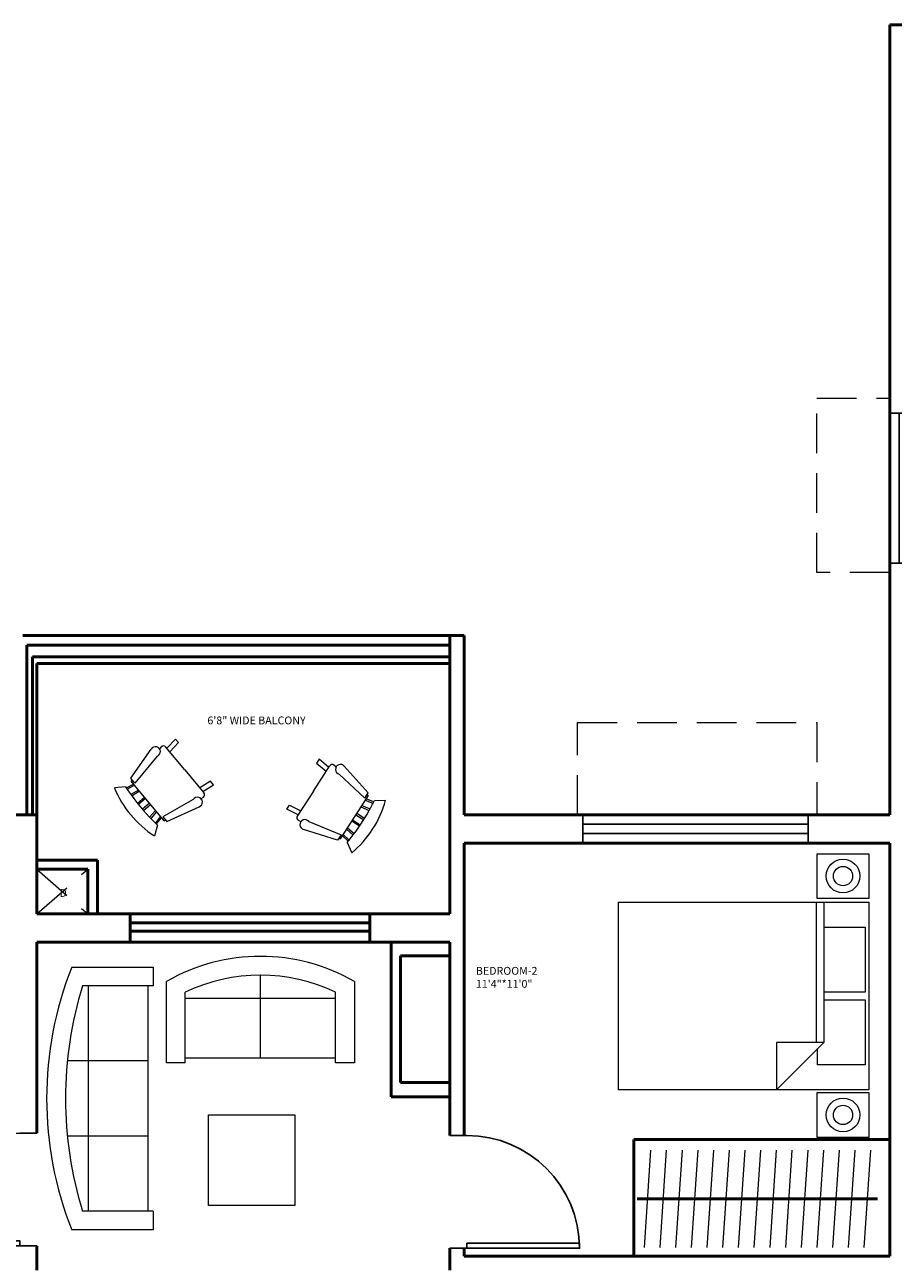
# Model space of a CAD drawing. Units: inches. Extents: x 291 to 2631, y 456 to 2623.
# Tile 16 of 22: x 1696 to 1974, y 2022 to 2418. Entities that reach past the tile are written whole.
import ezdxf

# ---------------------------------------------------------------- set-up
doc = ezdxf.new("R2010")
doc.units = ezdxf.units.IN
doc.linetypes.add('DASHED', pattern=[19.05, 12.7, -6.35])
for name, color, linetype, lineweight in [('A-ANNO-TEXT', 3, 'Continuous', 25), ('A-AREA-IDEN', 7, 'Continuous', 25), ('A-DOOR', 3, 'Continuous', 25), ('A-FLOR-OVHD', 1, 'DASHED', 18), ('A-FURN', 8, 'Continuous', 18), ('A-GLAZ', 4, 'Continuous', 25), ('A-WALL', 7, 'Continuous', 50)]:
    doc.layers.add(name, color=color, linetype=linetype, lineweight=lineweight)
doc.styles.get("Standard").update_dxf_attribs({"font": 'arial.ttf'})

# ---------------------------------------------------------------- blocks, each defined once
blk = doc.blocks.new('*U2')
for p, q in [((0, 0), (0, -6)), ((40, 0), (40, -6))]:
    blk.add_line(p, q)
blk.add_lwpolyline([(0, 0), (0, 40), (1.75, 40), (1.75, 0)], close=True)
blk.add_arc((0, 0), 40, 0, 90)
blk = doc.blocks.new('Bed - Queen')
for p, q in [((0, -80.00003), (0, 0)), ((0, 0), (59.99999, 0)), ((59.99999, 0), (59.99999, -80.00003)), ((7.99999, -1.2), (28.79998, -1.2)), ((7.99999, -14.4), (7.99999, -1.2)), ((28.79998, -1.2), (28.79998, -14.4)), ((31.19999, -1.2), (51.99999, -1.2)), ((31.19999, -14.4), (31.19999, -1.2)), ((51.99999, -1.2), (51.99999, -16.4)), ((0, -14.4), (44.8, -14.4)), ((59.99999, -29.6), (44.8, -14.4)), ((44.8, -14.4), (44.8, -29.6)), ((44.8, -16.8), (0, -16.8)), ((51.99999, -16.4), (46.79936, -16.4)), ((44.8, -29.6), (59.99999, -29.6)), ((59.99999, -80.00003), (0, -80.00003))]:
    blk.add_line(p, q)
blk = doc.blocks.new('Chair - Rocking')
for p, q in [((-8, -4.5), (-10, -1.5)), ((8, -4.5), (10, -1.5)), ((-9, -7.5), (-12, -18.49999)), ((-7, -7.5), (-9, -7.5)), ((-9, -18.49999), (-7, -7.5)), ((-8.23428, -6.99939), (-8.3093, -7.47958)), ((-8.23041, -7), (8.23915, -7)), ((-7.5, -4.5), (-7, -7)), ((-6.5, -7), (-7.02225, -4.43)), ((-4.5, -7), (-4.96674, -4.19951)), ((-4, -7), (-4.40532, -4.16272)), ((-1.5, -4.05012), (-1.5, -7)), ((-1, -7), (-1, -4.05012)), ((1, -7), (1, -4.04655)), ((1.5, -4.05012), (1.5, -7)), ((4, -7), (4.40187, -4.18694)), ((4.5, -7), (4.96761, -4.19437)), ((6.5, -7), (7, -4.4057)), ((7.5, -4.5), (7, -7)), ((7, -7.5), (9, -7.5)), ((9, -18.49999), (7, -7.5)), ((8.31071, -7.48854), (8.23449, -7.00073)), ((9, -7.5), (12, -18.49999)), ((-10.36644, -20.64523), (-10.5, -21.49999)), ((-9, -22.49999), (-9.5, -26.49999)), ((0, -22.49999), (-9.5, -22.49999)), ((-8, -26.49999), (-7.5, -22.49999)), ((0, -22.49999), (9.5, -22.49999)), ((8, -26.49999), (7.5, -22.49999)), ((9, -22.49999), (9.5, -26.49999)), ((10.5, -21.49999), (10.3575, -20.58798)), ((-9.5, -26.49999), (-8, -26.49999)), ((9.5, -26.49999), (8, -26.49999))]:
    blk.add_line(p, q)
for centre, radius, start, end in [((0, -34.08333), 34.08333, 72.93847, 107.0615), ((0, -68.25004), 64.25, 93.92211, 97.15267), ((0, -68.25004), 64.25, 82.84733, 93.92211), ((-10.5, -18.99999), 1.58114, 161.5651, 18.43495), ((10.5, -18.99999), 1.58114, 161.5651, 18.43495), ((-9.5, -21.49999), 1, 180, 270), ((9.5, -21.49999), 1, 270, 0)]:
    blk.add_arc(centre, radius, start, end)
blk = doc.blocks.new('Sofa - Roundback 7 ft.')
for p, q in [((-12.00002, -32.4421), (-12.00003, -6.5971)), ((11.99997, -32.4421), (11.99998, -6.5971)), ((-36.000027, -34), (-36.000027, -11.4696)), ((35.99998, -34), (35.99998, -11.4696)), ((-35.999844, -13.3819), (35.9998, -13.3819)), ((-36.000027, -32.4421), (35.99998, -32.4421))]:
    blk.add_line(p, q)
for points in [[(-36.000027, -34), (-42.000027, -34), (-42.000027, -8)], [(41.99998, -8), (41.99998, -34), (35.99998, -34)]]:
    blk.add_lwpolyline(points)
for centre, radius, start, end in [((0, -114.25), 114.25, 68.43141, 111.5686), ((-0.00001, -127.1968), 121.1968, 72.72033, 107.2797)]:
    blk.add_arc(centre, radius, start, end)
blk = doc.blocks.new('Sofa - Roundback Loveseat 5 ft.')
for p, q in [((0, -32.44198), (0, -5.99998)), ((-24, -33.99998), (-24, -11.46958)), ((24.00004, -33.99998), (24.00004, -11.46958)), ((-23.9998, -13.38178), (23.99986, -13.38178)), ((-24, -32.44198), (24.00004, -32.44198))]:
    blk.add_line(p, q)
for points in [[(-24, -33.99998), (-30, -33.99998), (-30, -7.99998)], [(30.00004, -7.99998), (30.00004, -33.99998), (24.00004, -33.99998)]]:
    blk.add_lwpolyline(points)
for centre, radius, start, end in [((0, -60.24998), 60.24998, 60.13715, 119.8628), ((0, -61.38438), 55.38444, 64.32083, 115.6792)]:
    blk.add_arc(centre, radius, start, end)
blk = doc.blocks.new('WIN-1800')
for p, q in [((0, 9), (72, 9)), ((0, 0), (0, 9)), ((72, 9), (72, 0)), ((0, 6), (72, 6)), ((72, 3), (0, 3)), ((72, 0), (0, 0))]:
    blk.add_line(p, q)
blk = doc.blocks.new('WIN-1200')
for p, q in [((0, 0), (0, 48)), ((0, 48), (9, 48)), ((3, 0), (3, 48)), ((6, 48), (6, 0)), ((9, 48), (9, 0)), ((9, 0), (0, 0))]:
    blk.add_line(p, q)

msp = doc.modelspace()

# ---------------------------------------------------------------- linework, layer by layer
at = {"layer": 'A-FLOR-OVHD'}
for p, q in [((1949.18, 2242.68), (1949.18, 2298.43)), ((1949.18, 2298.43), (1972.49, 2298.43)), ((1972.49, 2242.68), (1949.18, 2242.68)), ((1872.74, 2165.24), (1872.74, 2194.73)), ((1872.74, 2194.73), (1949.18, 2194.73)), ((1949.18, 2194.73), (1949.18, 2165.24)), ((1699.99, 2147.89), (1716.32, 2133.59)), ((1699.99, 2133.59), (1716.32, 2147.89))]:
    msp.add_line(p, q, dxfattribs=at)
at = {"layer": 'A-FURN'}
for p, q in [((1894.09, 2027.06), (1896.2, 2058.1)), ((1899.11, 2027.06), (1901.22, 2058.1)), ((1904.13, 2027.06), (1906.24, 2058.1)), ((1909.15, 2027.06), (1911.25, 2058.1)), ((1914.17, 2027.06), (1916.27, 2058.1)), ((1919.18, 2027.06), (1921.29, 2058.1)), ((1924.2, 2027.06), (1926.31, 2058.1)), ((1929.22, 2027.06), (1931.33, 2058.1)), ((1934.24, 2027.06), (1936.34, 2058.1)), ((1939.26, 2027.06), (1941.36, 2058.1)), ((1944.28, 2027.06), (1946.38, 2058.1)), ((1949.29, 2027.06), (1951.4, 2058.1)), ((1954.31, 2027.06), (1956.42, 2058.1)), ((1959.33, 2027.06), (1961.44, 2058.1)), ((1964.35, 2027.06), (1966.45, 2058.1))]:
    msp.add_line(p, q, dxfattribs=at)
for points in [[(1949.32, 2152.83), (1965.8, 2152.83), (1965.8, 2138.54), (1949.32, 2138.54)], [(1949.32, 2076.51), (1965.8, 2076.51), (1965.8, 2062.21), (1949.32, 2062.21)], [(1754.89, 2069.43), (1782.39, 2069.43), (1782.39, 2040.39), (1754.89, 2040.39)]]:
    msp.add_lwpolyline(points, close=True, dxfattribs=at)
for centre, radius in [((1957.56, 2145.69), 5.39), ((1957.56, 2145.69), 3.08), ((1957.56, 2069.36), 5.39), ((1957.56, 2069.36), 3.08)]:
    msp.add_circle(centre, radius, dxfattribs=at)
at = {"layer": 'A-WALL'}
for p, q in [((2059.49, 2417.68), (1972.49, 2417.68)), ((1972.49, 2417.68), (1972.49, 2165.24)), ((1695.49, 2222.59), (1699.99, 2222.59)), ((1699.99, 2222.59), (1831.99, 2222.59)), ((1836.49, 2222.59), (1831.99, 2222.59)), ((1831.99, 2165.24), (1831.99, 2222.59)), ((1836.49, 2165.24), (1836.49, 2222.59)), ((1696.8, 2165.24), (1696.8, 2219.47)), ((1696.8, 2219.47), (1831.99, 2219.47)), ((1698.62, 2165.24), (1698.62, 2215.78)), ((1698.62, 2215.78), (1831.99, 2215.78)), ((1699.99, 2213.59), (1831.99, 2213.59)), ((1699.99, 2213.59), (1699.99, 2165.24)), ((1699.99, 2165.24), (1554.49, 2165.24)), ((1699.99, 2165.24), (1699.99, 2133.59)), ((1831.99, 2165.24), (1831.99, 2133.59)), ((1972.49, 2165.24), (1836.49, 2165.24)), ((1972.49, 2156.24), (1836.49, 2156.24)), ((1836.49, 2156.24), (1836.49, 2062.78)), ((1972.49, 2156.24), (1972.49, 2024.24)), ((1699.99, 2150.74), (1719.39, 2150.74)), ((1719.39, 2150.74), (1719.39, 2133.59)), ((1699.99, 2147.89), (1716.32, 2147.89)), ((1716.32, 2147.89), (1716.32, 2133.59)), ((1699.99, 2133.59), (1831.99, 2133.59)), ((1729.85, 2133.59), (1729.85, 2124.59)), ((1806.39, 2133.59), (1806.39, 2124.59)), ((1729.85, 2130.75), (1806.39, 2130.75)), ((1729.85, 2128.07), (1806.39, 2128.07)), ((1699.99, 2124.59), (1831.99, 2124.59)), ((1699.99, 2124.59), (1699.99, 2063.53)), ((1813.18, 2075.12), (1813.18, 2124.59)), ((1831.99, 2124.59), (1831.99, 2062.78)), ((1831.99, 2120.21), (1816.19, 2120.21)), ((1816.19, 2120.21), (1816.19, 2079.78)), ((1816.19, 2079.78), (1831.99, 2079.78)), ((1813.18, 2075.12), (1831.99, 2075.12)), ((1890.73, 2024.24), (1890.73, 2061.49)), ((1890.73, 2061.49), (1972.49, 2061.49)), ((1891.78, 2042.58), (1968.58, 2042.58)), ((1699.99, 2027.53), (1699.99, 2019.74)), ((1831.99, 2026.78), (1831.99, 2019.74)), ((1836.49, 2026.78), (1836.49, 2024.24)), ((1972.49, 2024.24), (1836.49, 2024.24))]:
    msp.add_line(p, q, dxfattribs=at)

# ---------------------------------------------------------------- block references
at = {"layer": 'A-DOOR', "yscale": 0.9, "zscale": 0.9}
for p, xscale, rotation in [((1694.59, 2027.53), 0.9, 90), ((1837.39, 2026.78), -0.9, 270)]:
    msp.add_blockref('*U2', p, dxfattribs=dict(at, xscale=xscale, rotation=rotation))
at = {"layer": 'A-FURN'}
for name, p, rotation in [('Chair - Rocking', (1730.01, 2165.22), 129.7567937851614), ('Chair - Rocking', (1807.28, 2160.67), 237.1884930017563), ('Bed - Queen', (1965.86, 2137.35), 270), ('Sofa - Roundback 7 ft.', (1703.14, 2074.62), 90)]:
    msp.add_blockref(name, p, dxfattribs=dict(at, rotation=rotation))
msp.add_blockref('Sofa - Roundback Loveseat 5 ft.', (1771.44, 2120.02), dxfattribs=at)
at = {"layer": 'A-GLAZ'}
for name, p in [('WIN-1200', (1972.49, 2245.61)), ('WIN-1800', (1874.48, 2156.24))]:
    msp.add_blockref(name, p, dxfattribs=at)

# ---------------------------------------------------------------- texts
at = {"layer": 'A-ANNO-TEXT', "insert": (1707.23, 2141.55), "char_height": 2.5, "attachment_point": 1}
msp.add_mtext_dynamic_manual_height_columns('D', width=1.7946, gutter_width=12.5, heights=[0], dxfattribs=at)
at = {"layer": 'A-AREA-IDEN', "char_height": 2.5, "attachment_point": 1}
for s, width, insert in [('6\'8" WIDE BALCONY', 80.0851, (1754.5, 2196.67)), ('BEDROOM-2\\P11\'4"*11\'0"', 38.6939, (1840.27, 2116.66))]:
    msp.add_mtext_dynamic_manual_height_columns(s, width=width, gutter_width=12.5, heights=[0], dxfattribs=dict(at, insert=insert))

doc.saveas('drawing.dxf')
